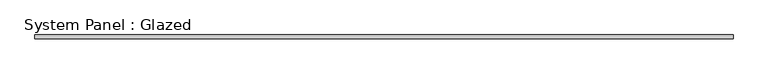
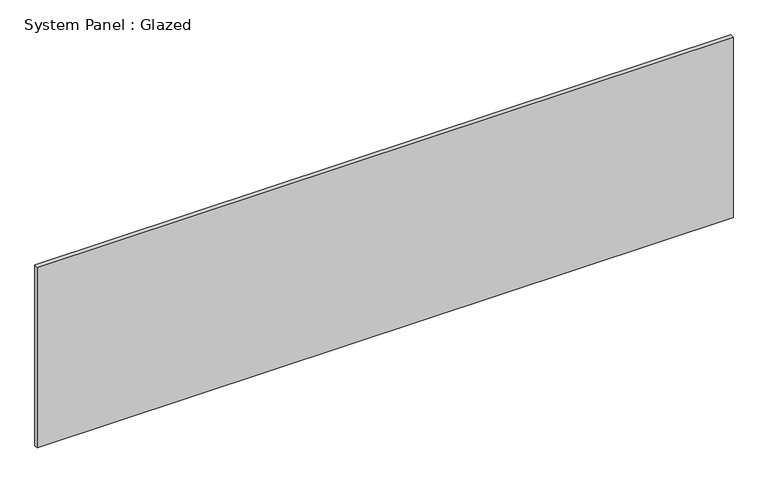
"""IFC4 building model written with IfcOpenShell, lengths in millimetres: plate geometry, System Panel : Glazed."""

from ifc_helpers import new_model, si_unit, origin, origin_with_axes, place, context, project, spatial, polyline, outline, extrude, source, transform, mapped, element, save


def system_panel_glazed_2b100c62(model_context):
    return source(origin(), model_context, "Body", "SweptSolid", [
        extrude(outline(polyline([(2279.65, 19.05), (-2279.65, 19.05), (-2279.65, 44.45), (2279.65, 44.45), (2279.65, 19.05)])), origin_with_axes(), (0.0, 0.0, 1.0), 1251.6739179),
    ])


if __name__ == "__main__":
    model = new_model("IFC4")
    model_context = context("Model", 3, world=origin())
    ifc_project = project(units=[si_unit("LENGTHUNIT", "METRE", prefix="MILLI")], contexts=[model_context])
    site = spatial("IfcSite", under=ifc_project)
    building = spatial("IfcBuilding", under=site)
    placement = place(None, origin())
    system_panel_glazed_shape = system_panel_glazed_2b100c62(model_context)
    element("IfcPlate", 1, ObjectType="System Panel : Glazed", at=placement, inside=building, context=model_context, shape_type="MappedRepresentation", body=[
        mapped(system_panel_glazed_shape, transform((0.0, 0.0, 0.0), x_axis=(1.0, 0.0, 0.0), y_axis=(0.0, 1.0, 0.0), z_axis=(0.0, 0.0, 1.0))),
    ])
    save(model, "model.ifc")

# Revit data of these elements
# Type "System Panel : Glazed"
#   Construction Type Id = "GSP4R"
#   Analytic Construction = "1/8 in Pilkington single glazing"
#   Visual Light Transmittance = 0.9
#   Solar Heat Gain Coefficient = 0.86
#   Heat Transfer Coefficient (U) = 1.18115 BTU/(h·ft²·°F)
#   Define Thermal Properties by = 1
# Element 1 (IfcPlate, "System Panel : Glazed")
#   Materials on its faces: "Glass"
# Materials
#   "Glass": class "Glass", colour RGB 0 128 192, transparency 0.75, Description = "Soda Lime Glass", Cost = 0
